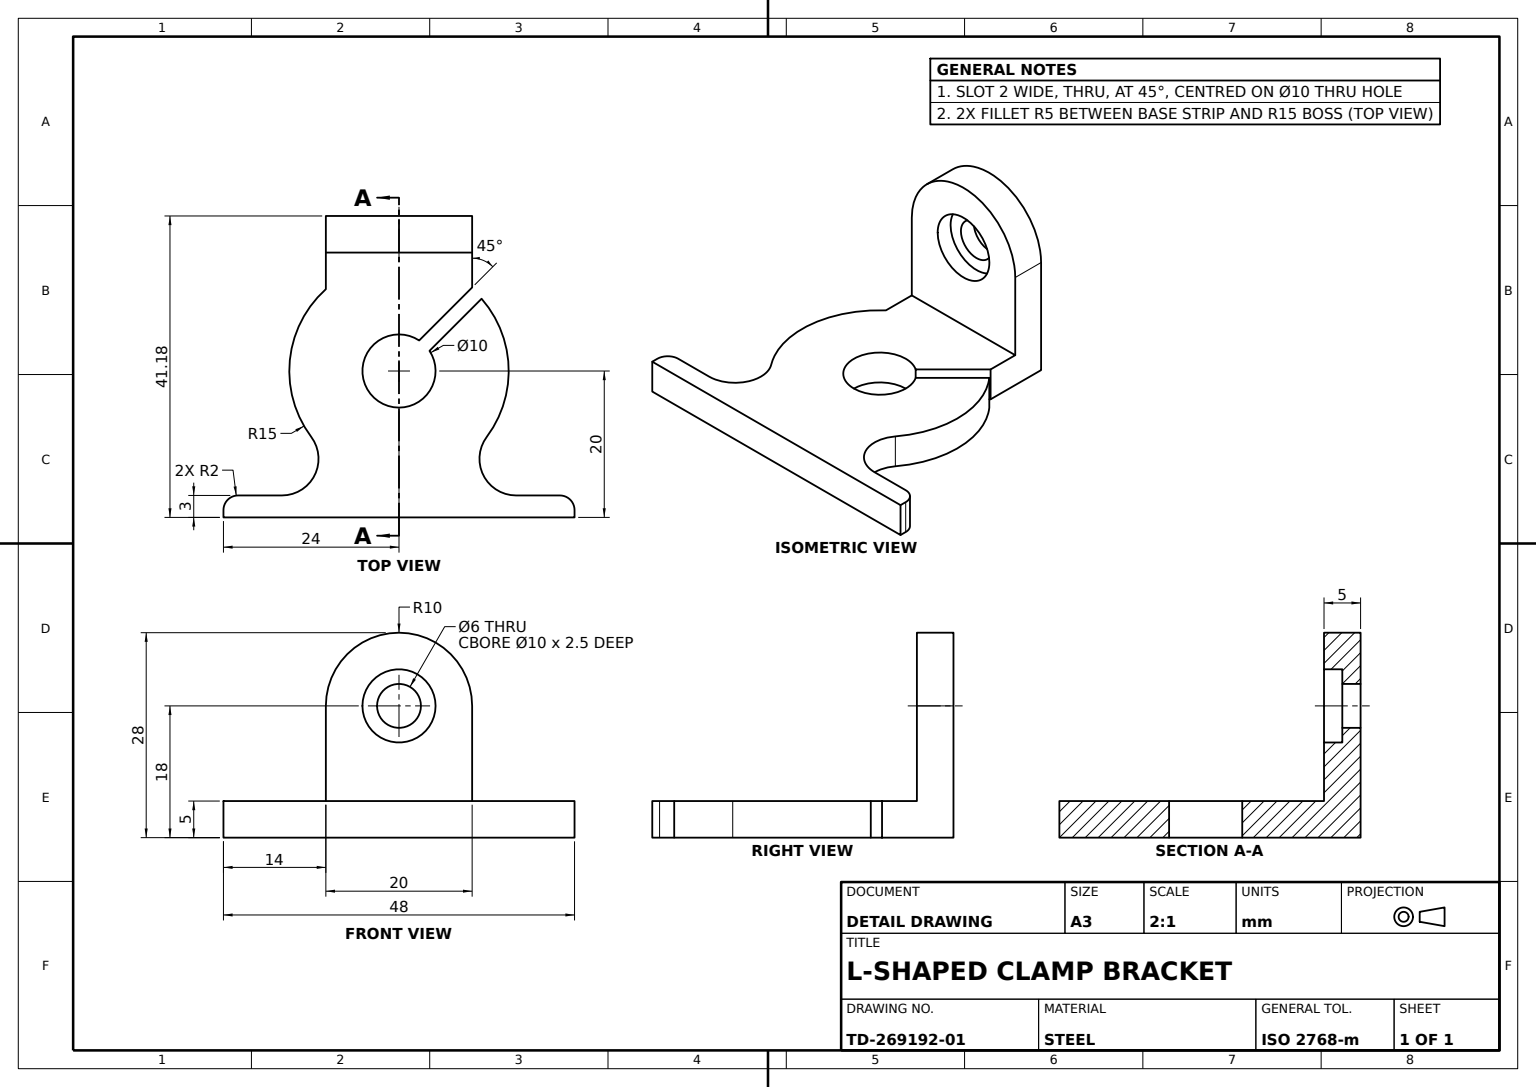
SolidWorks part; units mm, degrees
material "Plain Carbon Steel"
ref_plane "Front Plane" through (0, 0, 0) normal (0, 0, 1) x (1, 0, 0)
ref_plane "Top Plane" through (0, 0, 0) normal (0, 1, 0) x (1, 0, 0)
ref_plane "Right Plane" through (0, 0, 0) normal (1, 0, 0) x (0, 0, -1)
sketch "Base Plate Profile Sketch" plane through (0, 0, 0) normal (0, 1, 0) x (1, 0, 0)
  line L0 (-24, 0) -> (24, 0)
  line L1 (-24, 0) -> (-24, 1)
  line L2 (-22, 3) -> (-16, 3)
  line L3 (24, 1) -> (24, 0)
  line L4 (16, 3) -> (22, 3)
  line L6 (10, 31.4142) -> (10, 35)
  line L7 (-10, 31.1803) -> (-10, 35)
  line L8 (-10, 31.1803) -> (-10, 41.1803)
  line L9 (-10, 41.1803) -> (10, 41.1803)
  line L10 (10, 41.1803) -> (10, 31.4142)
  line L12 (4.1712, 22.757) -> (11.2901, 29.8759)
  line L14 (2.757, 24.1712) -> (10, 31.4142)
  arc A0 (2.757, 24.1712) -> (4.1712, 22.757) centre (0, 20) ccw
  arc A1 (12, 11) -> (11.2901, 29.8759) centre (0, 20) ccw
  arc A2 (-12, 11) -> (-16, 3) centre (-16, 8) cw
  arc A3 (12, 11) -> (16, 3) centre (16, 8) ccw
  arc A4 (-24, 1) -> (-22, 3) centre (-22, 1) cw
  arc A5 (22, 3) -> (24, 1) centre (22, 1) cw
  arc A6 (-10, 31.1803) -> (-12, 11) centre (0, 20) ccw
  arc A7 (-10, 31.1803) -> (-12, 11) centre (0, 20) ccw
  arc A8 (12, 11) -> (11.2901, 29.8759) centre (0, 20) ccw
  point P4 (0, 0)
  point P18 (24, 3)
  point P19 (0, 0)
  point P20 (0, 35)
  point P23 (-10, 0)
  point P28 (0.7071, 19.2929)
  point P30 (22.8088, 42.8088)
  point P31 (23.5159, 42.1017)
  point P32 (-0.7071, 20.7071)
  point P33 (22.1017, 43.5159)
  dimension "D1" = 10
  dimension "D2" = 30
  dimension "D7" = 5
  dimension "D8" = 5
  dimension "D9" = 2
  dimension "D13" = 0.7071
  dimension "D3" = 48
  dimension "D4" = 3
  dimension "D5" = 17
  dimension "D6" = 20
  dimension "D10" = 10
  dimension "D12" = 35
  dimension "D11" = 20
  dimension "D14" = 0.7071
  dimension "D15" = 0.7071
  dimension "D16" = 0.7071
  dimension "D17" = 9.7661
  dimension "D18" = 45
  dimension "D19" = 10
extrude "Base Plate 5mm" add sketch "Base Plate Profile Sketch" along normal blind 5 contours L7 A6 A2 L2 A4 L1 L0 L3 A5 L4 A3 A1 L12 A0 L14 L6 L10 L9 L8
sketch "Upright Lug Profile Sketch" plane through (0, 0, -41.1803) normal (0, 0, -1) x (-1, 0, 0)
  line L0 (-10, 18) -> (-10, 0)
  line L1 (-10, 0) -> (10, 0)
  line L2 (10, 5) -> (10, 0) construction
  line L3 (10, 0) -> (-10, 0) construction
  line L4 (10, 0) -> (10, 18)
  arc A0 (10, 18) -> (-10, 18) centre (0, 18) ccw
  circle A1 centre (0, 18) radius 3
  dimension "D1" = 20
  dimension "D2" = 6
  dimension "D3" = 18
  dimension "D4" = 18
extrude "Upright Lug" add sketch "Upright Lug Profile Sketch" against normal blind 5
sketch "Pivot Counterbore Sketch" plane through (0, 0, -36.1803) normal (0, 0, 1) x (1, 0, 0)
  circle A0 centre (0, 18) radius 3
  circle A1 centre (0, 18) radius 5
  dimension "D1" = 6
  dimension "D2" = 10
extrude "Pivot Counterbore Ø10x2.5" cut sketch "Pivot Counterbore Sketch" against normal blind 2.5
